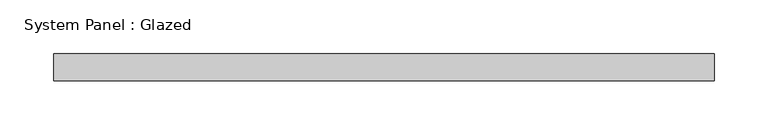
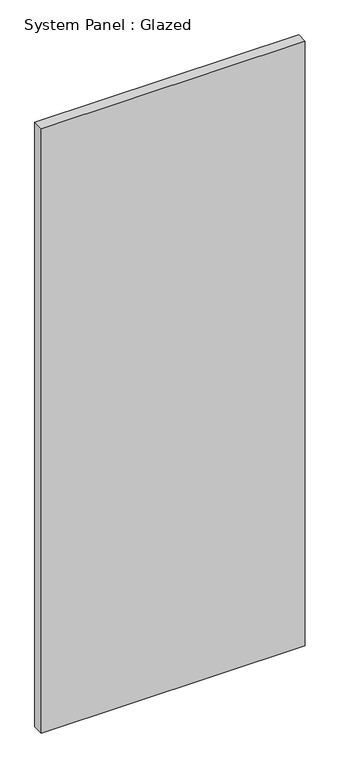
"""IFC4 building model written with IfcOpenShell, lengths in millimetres: plate geometry, System Panel : Glazed."""

from ifc_helpers import new_model, si_unit, origin, origin_with_axes, place, context, project, spatial, polyline, outline, extrude, source, transform, mapped, element, save


def system_panel_glazed_6ea480bf(model_context):
    return source(origin(), model_context, "Body", "SweptSolid", [
        extrude(outline(polyline([(307.975, 19.05), (-307.975, 19.05), (-307.975, 44.45), (307.975, 44.45), (307.975, 19.05)])), origin_with_axes(), (0.0, 0.0, 1.0), 1490.4100631),
    ])


if __name__ == "__main__":
    model = new_model("IFC4")
    model_context = context("Model", 3, world=origin())
    ifc_project = project(units=[si_unit("LENGTHUNIT", "METRE", prefix="MILLI")], contexts=[model_context])
    site = spatial("IfcSite", under=ifc_project)
    building = spatial("IfcBuilding", under=site)
    placement = place(None, origin())
    system_panel_glazed_shape = system_panel_glazed_6ea480bf(model_context)
    element("IfcPlate", 1, ObjectType="System Panel : Glazed", at=placement, inside=building, context=model_context, shape_type="MappedRepresentation", body=[
        mapped(system_panel_glazed_shape, transform((0.0, 0.0, 0.0), x_axis=(1.0, 0.0, 0.0), y_axis=(0.0, 1.0, 0.0), z_axis=(0.0, 0.0, 1.0))),
    ])
    save(model, "model.ifc")

# Revit data of these elements
# Type "System Panel : Glazed"
#   Construction Type Id = "GSP4R"
#   Analytic Construction = "1/8 in Pilkington single glazing"
#   Visual Light Transmittance = 0.9
#   Solar Heat Gain Coefficient = 0.86
#   Heat Transfer Coefficient (U) = 1.18115 BTU/(h·ft²·°F)
#   Define Thermal Properties by = 1
# Element 1 (IfcPlate, "System Panel : Glazed")
#   Materials on its faces: "Glass"
# Materials
#   "Glass": class "Glass", colour RGB 0 128 192, transparency 0.75, Description = "Soda Lime Glass", Cost = 0
